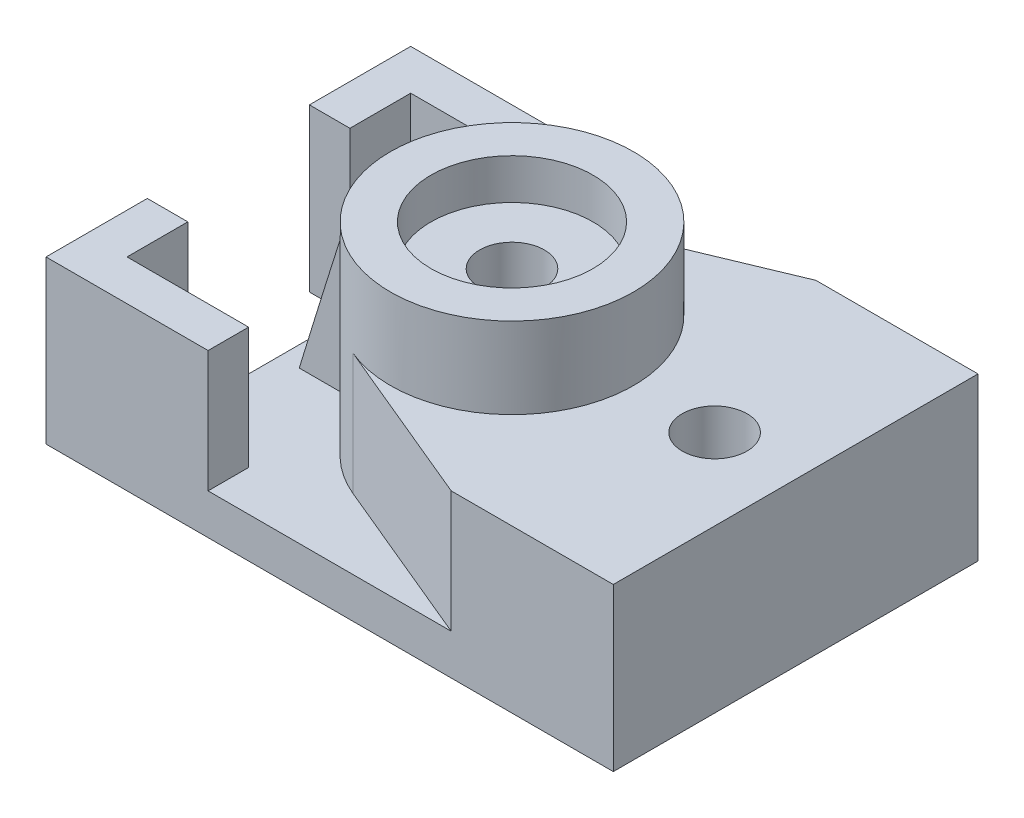
ISO-10303-21;
HEADER;
FILE_DESCRIPTION(('STEP AP214'),'2;1');
FILE_NAME('part.step','',(''),(''),'','','');
FILE_SCHEMA(('AUTOMOTIVE_DESIGN { 1 0 10303 214 1 1 1 1 }'));
ENDSEC;
DATA;
#1=APPLICATION_CONTEXT('core data for automotive mechanical design processes');
#2=APPLICATION_PROTOCOL_DEFINITION('international standard','automotive_design',2000,#1);
#3=PRODUCT_CONTEXT('',#1,'mechanical');
#4=PRODUCT('Part','Part','',(#3));
#5=PRODUCT_RELATED_PRODUCT_CATEGORY('part','',(#4));
#6=PRODUCT_DEFINITION_FORMATION('','',#4);
#7=PRODUCT_DEFINITION_CONTEXT('part definition',#1,'design');
#8=PRODUCT_DEFINITION('design','',#6,#7);
#9=PRODUCT_DEFINITION_SHAPE('','',#8);
#10=(LENGTH_UNIT() NAMED_UNIT(*) SI_UNIT(.MILLI.,.METRE.));
#11=(NAMED_UNIT(*) PLANE_ANGLE_UNIT() SI_UNIT($,.RADIAN.));
#12=(NAMED_UNIT(*) SI_UNIT($,.STERADIAN.) SOLID_ANGLE_UNIT());
#13=UNCERTAINTY_MEASURE_WITH_UNIT(LENGTH_MEASURE(1.E-05),#10,'distance_accuracy_value','');
#14=(GEOMETRIC_REPRESENTATION_CONTEXT(3) GLOBAL_UNCERTAINTY_ASSIGNED_CONTEXT((#13)) GLOBAL_UNIT_ASSIGNED_CONTEXT((#10,
#11,#12)) REPRESENTATION_CONTEXT('',''));
#15=CARTESIAN_POINT('',(0.,0.,0.));
#16=DIRECTION('',(0.,0.,1.));
#17=DIRECTION('',(1.,0.,0.));
#18=AXIS2_PLACEMENT_3D('',#15,#16,#17);
#19=CARTESIAN_POINT('',(-70.,40.,45.));
#20=DIRECTION('',(1.,0.,0.));
#21=DIRECTION('',(0.,0.,-1.));
#22=AXIS2_PLACEMENT_3D('',#19,#20,#21);
#23=PLANE('',#22);
#24=DIRECTION('',(0.,0.,1.));
#25=VECTOR('',#24,1.);
#26=CARTESIAN_POINT('',(-70.,0.,45.));
#27=LINE('',#26,#25);
#28=CARTESIAN_POINT('',(-70.,0.,-45.));
#29=VERTEX_POINT('',#28);
#30=CARTESIAN_POINT('',(-70.,0.,-20.));
#31=VERTEX_POINT('',#30);
#32=EDGE_CURVE('E422',#29,#31,#27,.T.);
#33=ORIENTED_EDGE('',*,*,#32,.T.);
#34=DIRECTION('',(0.,1.,0.));
#35=VECTOR('',#34,1.);
#36=CARTESIAN_POINT('',(-70.,10.,-20.));
#37=LINE('',#36,#35);
#38=CARTESIAN_POINT('',(-70.,40.,-20.));
#39=VERTEX_POINT('',#38);
#40=EDGE_CURVE('E365',#31,#39,#37,.T.);
#41=ORIENTED_EDGE('',*,*,#40,.T.);
#42=DIRECTION('',(0.,0.,1.));
#43=VECTOR('',#42,1.);
#44=CARTESIAN_POINT('',(-70.,40.,45.));
#45=LINE('',#44,#43);
#46=CARTESIAN_POINT('',(-70.,40.,-45.));
#47=VERTEX_POINT('',#46);
#48=EDGE_CURVE('E409',#47,#39,#45,.T.);
#49=ORIENTED_EDGE('',*,*,#48,.F.);
#50=DIRECTION('',(0.,-1.,0.));
#51=VECTOR('',#50,1.);
#52=CARTESIAN_POINT('',(-70.,40.,-45.));
#53=LINE('',#52,#51);
#54=EDGE_CURVE('E431',#47,#29,#53,.T.);
#55=ORIENTED_EDGE('',*,*,#54,.T.);
#56=EDGE_LOOP('',(#33,#41,#49,#55));
#57=FACE_BOUND('',#56,.T.);
#58=ADVANCED_FACE('F55',(#57),#23,.F.);
#59=CARTESIAN_POINT('',(0.,40.,0.));
#60=DIRECTION('',(0.,-1.,0.));
#61=DIRECTION('',(0.,0.,-1.));
#62=AXIS2_PLACEMENT_3D('',#59,#60,#61);
#63=PLANE('',#62);
#64=ORIENTED_EDGE('',*,*,#48,.T.);
#65=DIRECTION('',(-1.,0.,0.));
#66=VECTOR('',#65,1.);
#67=CARTESIAN_POINT('',(-70.,40.,-20.));
#68=LINE('',#67,#66);
#69=CARTESIAN_POINT('',(-60.,40.,-20.));
#70=VERTEX_POINT('',#69);
#71=EDGE_CURVE('E313',#70,#39,#68,.T.);
#72=ORIENTED_EDGE('',*,*,#71,.F.);
#73=DIRECTION('',(0.,0.,1.));
#74=VECTOR('',#73,1.);
#75=CARTESIAN_POINT('',(-60.,40.,-20.));
#76=LINE('',#75,#74);
#77=CARTESIAN_POINT('',(-60.,40.,-35.));
#78=VERTEX_POINT('',#77);
#79=EDGE_CURVE('E356',#78,#70,#76,.T.);
#80=ORIENTED_EDGE('',*,*,#79,.F.);
#81=DIRECTION('',(-1.,0.,0.));
#82=VECTOR('',#81,1.);
#83=CARTESIAN_POINT('',(-60.,40.,-35.));
#84=LINE('',#83,#82);
#85=CARTESIAN_POINT('',(-30.,40.,-35.));
#86=VERTEX_POINT('',#85);
#87=EDGE_CURVE('E351',#86,#78,#84,.T.);
#88=ORIENTED_EDGE('',*,*,#87,.F.);
#89=DIRECTION('',(0.,0.,1.));
#90=VECTOR('',#89,1.);
#91=CARTESIAN_POINT('',(-30.,40.,-35.));
#92=LINE('',#91,#90);
#93=CARTESIAN_POINT('',(-30.,40.,-45.));
#94=VERTEX_POINT('',#93);
#95=EDGE_CURVE('E355',#94,#86,#92,.T.);
#96=ORIENTED_EDGE('',*,*,#95,.F.);
#97=DIRECTION('',(-1.,0.,0.));
#98=VECTOR('',#97,1.);
#99=CARTESIAN_POINT('',(-70.,40.,-45.));
#100=LINE('',#99,#98);
#101=EDGE_CURVE('E405',#94,#47,#100,.T.);
#102=ORIENTED_EDGE('',*,*,#101,.T.);
#103=EDGE_LOOP('',(#64,#72,#80,#88,#96,#102));
#104=FACE_BOUND('',#103,.T.);
#105=ADVANCED_FACE('F453',(#104),#63,.F.);
#106=CARTESIAN_POINT('',(50.,40.,0.));
#107=DIRECTION('',(0.,1.,0.));
#108=DIRECTION('',(0.,0.,1.));
#109=AXIS2_PLACEMENT_3D('',#106,#107,#108);
#110=CIRCLE('',#109,8.);
#111=CARTESIAN_POINT('',(50.,40.,8.));
#112=VERTEX_POINT('',#111);
#113=EDGE_CURVE('E285',#112,#112,#110,.T.);
#114=ORIENTED_EDGE('',*,*,#113,.F.);
#115=EDGE_LOOP('',(#114));
#116=FACE_BOUND('',#115,.T.);
#117=CARTESIAN_POINT('',(70.,40.,-45.));
#118=VERTEX_POINT('',#117);
#119=CARTESIAN_POINT('',(30.,40.,-45.));
#120=VERTEX_POINT('',#119);
#121=EDGE_CURVE('E404',#118,#120,#100,.T.);
#122=ORIENTED_EDGE('',*,*,#121,.T.);
#123=DIRECTION('',(0.923076923076923,0.,-0.384615384615384));
#124=VECTOR('',#123,1.);
#125=CARTESIAN_POINT('',(-11.5384615384615,40.,-27.6923076923077));
#126=LINE('',#125,#124);
#127=CARTESIAN_POINT('',(-11.5384615384615,40.,-27.6923076923077));
#128=VERTEX_POINT('',#127);
#129=EDGE_CURVE('E348',#128,#120,#126,.T.);
#130=ORIENTED_EDGE('',*,*,#129,.F.);
#131=CARTESIAN_POINT('',(0.,40.,0.));
#132=DIRECTION('',(0.,-1.,0.));
#133=DIRECTION('',(0.,0.,-1.));
#134=AXIS2_PLACEMENT_3D('',#131,#132,#133);
#135=CIRCLE('',#134,30.);
#136=CARTESIAN_POINT('',(-11.5384615384615,40.,27.6923076923077));
#137=VERTEX_POINT('',#136);
#138=EDGE_CURVE('E393',#137,#128,#135,.F.);
#139=ORIENTED_EDGE('',*,*,#138,.F.);
#140=DIRECTION('',(-0.923076923076923,0.,-0.384615384615384));
#141=VECTOR('',#140,1.);
#142=CARTESIAN_POINT('',(-11.5384615384615,40.,27.6923076923077));
#143=LINE('',#142,#141);
#144=CARTESIAN_POINT('',(30.,40.,45.));
#145=VERTEX_POINT('',#144);
#146=EDGE_CURVE('E349',#145,#137,#143,.T.);
#147=ORIENTED_EDGE('',*,*,#146,.F.);
#148=DIRECTION('',(1.,0.,0.));
#149=VECTOR('',#148,1.);
#150=CARTESIAN_POINT('',(-70.,40.,45.));
#151=LINE('',#150,#149);
#152=CARTESIAN_POINT('',(70.,40.,45.));
#153=VERTEX_POINT('',#152);
#154=EDGE_CURVE('E412',#145,#153,#151,.T.);
#155=ORIENTED_EDGE('',*,*,#154,.T.);
#156=DIRECTION('',(0.,0.,-1.));
#157=VECTOR('',#156,1.);
#158=CARTESIAN_POINT('',(70.,40.,45.));
#159=LINE('',#158,#157);
#160=EDGE_CURVE('E399',#153,#118,#159,.T.);
#161=ORIENTED_EDGE('',*,*,#160,.T.);
#162=EDGE_LOOP('',(#122,#130,#139,#147,#155,#161));
#163=FACE_BOUND('',#162,.T.);
#164=ADVANCED_FACE('F467',(#116,#163),#63,.F.);
#165=CARTESIAN_POINT('',(70.,40.,45.));
#166=DIRECTION('',(-1.,0.,0.));
#167=DIRECTION('',(0.,0.,1.));
#168=AXIS2_PLACEMENT_3D('',#165,#166,#167);
#169=PLANE('',#168);
#170=DIRECTION('',(0.,0.,-1.));
#171=VECTOR('',#170,1.);
#172=CARTESIAN_POINT('',(70.,0.,45.));
#173=LINE('',#172,#171);
#174=CARTESIAN_POINT('',(70.,0.,45.));
#175=VERTEX_POINT('',#174);
#176=CARTESIAN_POINT('',(70.,0.,-45.));
#177=VERTEX_POINT('',#176);
#178=EDGE_CURVE('E417',#175,#177,#173,.T.);
#179=ORIENTED_EDGE('',*,*,#178,.T.);
#180=DIRECTION('',(0.,-1.,0.));
#181=VECTOR('',#180,1.);
#182=CARTESIAN_POINT('',(70.,40.,-45.));
#183=LINE('',#182,#181);
#184=EDGE_CURVE('E398',#118,#177,#183,.T.);
#185=ORIENTED_EDGE('',*,*,#184,.F.);
#186=ORIENTED_EDGE('',*,*,#160,.F.);
#187=DIRECTION('',(0.,-1.,0.));
#188=VECTOR('',#187,1.);
#189=CARTESIAN_POINT('',(70.,40.,45.));
#190=LINE('',#189,#188);
#191=EDGE_CURVE('E413',#153,#175,#190,.T.);
#192=ORIENTED_EDGE('',*,*,#191,.T.);
#193=EDGE_LOOP('',(#179,#185,#186,#192));
#194=FACE_BOUND('',#193,.T.);
#195=ADVANCED_FACE('F53',(#194),#169,.F.);
#196=CARTESIAN_POINT('',(-70.,40.,-45.));
#197=DIRECTION('',(0.,0.,1.));
#198=DIRECTION('',(1.,0.,0.));
#199=AXIS2_PLACEMENT_3D('',#196,#197,#198);
#200=PLANE('',#199);
#201=ORIENTED_EDGE('',*,*,#101,.F.);
#202=DIRECTION('',(0.,1.,0.));
#203=VECTOR('',#202,1.);
#204=CARTESIAN_POINT('',(-30.,10.,-45.));
#205=LINE('',#204,#203);
#206=CARTESIAN_POINT('',(-30.,10.,-45.));
#207=VERTEX_POINT('',#206);
#208=EDGE_CURVE('E375',#207,#94,#205,.T.);
#209=ORIENTED_EDGE('',*,*,#208,.F.);
#210=DIRECTION('',(-1.,0.,0.));
#211=VECTOR('',#210,1.);
#212=CARTESIAN_POINT('',(-30.,10.,-45.));
#213=LINE('',#212,#211);
#214=CARTESIAN_POINT('',(30.,10.,-45.));
#215=VERTEX_POINT('',#214);
#216=EDGE_CURVE('E323',#215,#207,#213,.T.);
#217=ORIENTED_EDGE('',*,*,#216,.F.);
#218=DIRECTION('',(0.,1.,0.));
#219=VECTOR('',#218,1.);
#220=CARTESIAN_POINT('',(30.,10.,-45.));
#221=LINE('',#220,#219);
#222=EDGE_CURVE('E372',#215,#120,#221,.T.);
#223=ORIENTED_EDGE('',*,*,#222,.T.);
#224=ORIENTED_EDGE('',*,*,#121,.F.);
#225=ORIENTED_EDGE('',*,*,#184,.T.);
#226=DIRECTION('',(-1.,0.,0.));
#227=VECTOR('',#226,1.);
#228=CARTESIAN_POINT('',(-70.,0.,-45.));
#229=LINE('',#228,#227);
#230=EDGE_CURVE('E419',#177,#29,#229,.T.);
#231=ORIENTED_EDGE('',*,*,#230,.T.);
#232=ORIENTED_EDGE('',*,*,#54,.F.);
#233=EDGE_LOOP('',(#201,#209,#217,#223,#224,#225,#231,#232));
#234=FACE_BOUND('',#233,.T.);
#235=ADVANCED_FACE('F440',(#234),#200,.F.);
#236=DIRECTION('',(0.,1.,0.));
#237=VECTOR('',#236,1.);
#238=CARTESIAN_POINT('',(-70.,10.,20.));
#239=LINE('',#238,#237);
#240=CARTESIAN_POINT('',(-70.,0.,20.));
#241=VERTEX_POINT('',#240);
#242=CARTESIAN_POINT('',(-70.,40.,20.));
#243=VERTEX_POINT('',#242);
#244=EDGE_CURVE('E340',#241,#243,#239,.T.);
#245=ORIENTED_EDGE('',*,*,#244,.F.);
#246=CARTESIAN_POINT('',(-70.,0.,45.));
#247=VERTEX_POINT('',#246);
#248=EDGE_CURVE('E423',#241,#247,#27,.T.);
#249=ORIENTED_EDGE('',*,*,#248,.T.);
#250=DIRECTION('',(0.,-1.,0.));
#251=VECTOR('',#250,1.);
#252=CARTESIAN_POINT('',(-70.,40.,45.));
#253=LINE('',#252,#251);
#254=CARTESIAN_POINT('',(-70.,40.,45.));
#255=VERTEX_POINT('',#254);
#256=EDGE_CURVE('E426',#255,#247,#253,.T.);
#257=ORIENTED_EDGE('',*,*,#256,.F.);
#258=EDGE_CURVE('E410',#243,#255,#45,.T.);
#259=ORIENTED_EDGE('',*,*,#258,.F.);
#260=EDGE_LOOP('',(#245,#249,#257,#259));
#261=FACE_BOUND('',#260,.T.);
#262=ADVANCED_FACE('F480',(#261),#23,.F.);
#263=CARTESIAN_POINT('',(-70.,40.,45.));
#264=DIRECTION('',(0.,0.,-1.));
#265=DIRECTION('',(-1.,0.,0.));
#266=AXIS2_PLACEMENT_3D('',#263,#264,#265);
#267=PLANE('',#266);
#268=ORIENTED_EDGE('',*,*,#154,.F.);
#269=DIRECTION('',(0.,1.,0.));
#270=VECTOR('',#269,1.);
#271=CARTESIAN_POINT('',(30.,10.,45.));
#272=LINE('',#271,#270);
#273=CARTESIAN_POINT('',(30.,10.,45.));
#274=VERTEX_POINT('',#273);
#275=EDGE_CURVE('E382',#274,#145,#272,.T.);
#276=ORIENTED_EDGE('',*,*,#275,.F.);
#277=DIRECTION('',(1.,0.,0.));
#278=VECTOR('',#277,1.);
#279=CARTESIAN_POINT('',(-30.,10.,45.));
#280=LINE('',#279,#278);
#281=CARTESIAN_POINT('',(-30.,10.,45.));
#282=VERTEX_POINT('',#281);
#283=EDGE_CURVE('E318',#282,#274,#280,.T.);
#284=ORIENTED_EDGE('',*,*,#283,.F.);
#285=DIRECTION('',(0.,1.,0.));
#286=VECTOR('',#285,1.);
#287=CARTESIAN_POINT('',(-30.,10.,45.));
#288=LINE('',#287,#286);
#289=CARTESIAN_POINT('',(-30.,40.,45.));
#290=VERTEX_POINT('',#289);
#291=EDGE_CURVE('E384',#282,#290,#288,.T.);
#292=ORIENTED_EDGE('',*,*,#291,.T.);
#293=EDGE_CURVE('E415',#255,#290,#151,.T.);
#294=ORIENTED_EDGE('',*,*,#293,.F.);
#295=ORIENTED_EDGE('',*,*,#256,.T.);
#296=DIRECTION('',(1.,0.,0.));
#297=VECTOR('',#296,1.);
#298=CARTESIAN_POINT('',(-70.,0.,45.));
#299=LINE('',#298,#297);
#300=EDGE_CURVE('E401',#247,#175,#299,.T.);
#301=ORIENTED_EDGE('',*,*,#300,.T.);
#302=ORIENTED_EDGE('',*,*,#191,.F.);
#303=EDGE_LOOP('',(#268,#276,#284,#292,#294,#295,#301,#302));
#304=FACE_BOUND('',#303,.T.);
#305=ADVANCED_FACE('F475',(#304),#267,.F.);
#306=ORIENTED_EDGE('',*,*,#293,.T.);
#307=DIRECTION('',(0.,0.,1.));
#308=VECTOR('',#307,1.);
#309=CARTESIAN_POINT('',(-30.,40.,35.));
#310=LINE('',#309,#308);
#311=CARTESIAN_POINT('',(-30.,40.,35.));
#312=VERTEX_POINT('',#311);
#313=EDGE_CURVE('E347',#312,#290,#310,.T.);
#314=ORIENTED_EDGE('',*,*,#313,.F.);
#315=DIRECTION('',(1.,0.,0.));
#316=VECTOR('',#315,1.);
#317=CARTESIAN_POINT('',(-60.,40.,35.));
#318=LINE('',#317,#316);
#319=CARTESIAN_POINT('',(-60.,40.,35.));
#320=VERTEX_POINT('',#319);
#321=EDGE_CURVE('E344',#320,#312,#318,.T.);
#322=ORIENTED_EDGE('',*,*,#321,.F.);
#323=DIRECTION('',(0.,0.,1.));
#324=VECTOR('',#323,1.);
#325=CARTESIAN_POINT('',(-60.,40.,20.));
#326=LINE('',#325,#324);
#327=CARTESIAN_POINT('',(-60.,40.,20.));
#328=VERTEX_POINT('',#327);
#329=EDGE_CURVE('E338',#328,#320,#326,.T.);
#330=ORIENTED_EDGE('',*,*,#329,.F.);
#331=DIRECTION('',(1.,0.,0.));
#332=VECTOR('',#331,1.);
#333=CARTESIAN_POINT('',(-70.,40.,20.));
#334=LINE('',#333,#332);
#335=EDGE_CURVE('E307',#243,#328,#334,.T.);
#336=ORIENTED_EDGE('',*,*,#335,.F.);
#337=ORIENTED_EDGE('',*,*,#258,.T.);
#338=EDGE_LOOP('',(#306,#314,#322,#330,#336,#337));
#339=FACE_BOUND('',#338,.T.);
#340=ADVANCED_FACE('F513',(#339),#63,.F.);
#341=CARTESIAN_POINT('',(0.,0.,0.));
#342=DIRECTION('',(0.,-1.,0.));
#343=DIRECTION('',(0.,0.,-1.));
#344=AXIS2_PLACEMENT_3D('',#341,#342,#343);
#345=PLANE('',#344);
#346=DIRECTION('',(-1.,0.,0.));
#347=VECTOR('',#346,1.);
#348=CARTESIAN_POINT('',(-70.,0.,-20.));
#349=LINE('',#348,#347);
#350=CARTESIAN_POINT('',(-50.,0.,-20.));
#351=VERTEX_POINT('',#350);
#352=EDGE_CURVE('E295',#351,#31,#349,.T.);
#353=ORIENTED_EDGE('',*,*,#352,.T.);
#354=ORIENTED_EDGE('',*,*,#32,.F.);
#355=ORIENTED_EDGE('',*,*,#230,.F.);
#356=ORIENTED_EDGE('',*,*,#178,.F.);
#357=ORIENTED_EDGE('',*,*,#300,.F.);
#358=ORIENTED_EDGE('',*,*,#248,.F.);
#359=DIRECTION('',(1.,0.,0.));
#360=VECTOR('',#359,1.);
#361=CARTESIAN_POINT('',(-70.,0.,20.));
#362=LINE('',#361,#360);
#363=CARTESIAN_POINT('',(-50.,0.,20.));
#364=VERTEX_POINT('',#363);
#365=EDGE_CURVE('E288',#241,#364,#362,.T.);
#366=ORIENTED_EDGE('',*,*,#365,.T.);
#367=DIRECTION('',(0.,0.,-1.));
#368=VECTOR('',#367,1.);
#369=CARTESIAN_POINT('',(-50.,0.,-20.));
#370=LINE('',#369,#368);
#371=EDGE_CURVE('E293',#364,#351,#370,.T.);
#372=ORIENTED_EDGE('',*,*,#371,.T.);
#373=EDGE_LOOP('',(#353,#354,#355,#356,#357,#358,#366,#372));
#374=FACE_BOUND('',#373,.T.);
#375=CARTESIAN_POINT('',(50.,0.,0.));
#376=DIRECTION('',(0.,-1.,0.));
#377=DIRECTION('',(0.,0.,-1.));
#378=AXIS2_PLACEMENT_3D('',#375,#376,#377);
#379=CIRCLE('',#378,8.);
#380=CARTESIAN_POINT('',(50.,0.,-8.));
#381=VERTEX_POINT('',#380);
#382=EDGE_CURVE('E287',#381,#381,#379,.F.);
#383=ORIENTED_EDGE('',*,*,#382,.T.);
#384=EDGE_LOOP('',(#383));
#385=FACE_BOUND('',#384,.T.);
#386=CARTESIAN_POINT('',(0.,0.,0.));
#387=DIRECTION('',(0.,-1.,0.));
#388=DIRECTION('',(0.,0.,-1.));
#389=AXIS2_PLACEMENT_3D('',#386,#387,#388);
#390=CIRCLE('',#389,8.);
#391=CARTESIAN_POINT('',(0.,0.,-8.));
#392=VERTEX_POINT('',#391);
#393=EDGE_CURVE('E283',#392,#392,#390,.F.);
#394=ORIENTED_EDGE('',*,*,#393,.T.);
#395=EDGE_LOOP('',(#394));
#396=FACE_BOUND('',#395,.T.);
#397=ADVANCED_FACE('F444',(#374,#385,#396),#345,.T.);
#398=CARTESIAN_POINT('',(0.,60.,0.));
#399=DIRECTION('',(0.,-1.,0.));
#400=DIRECTION('',(0.,0.,-1.));
#401=AXIS2_PLACEMENT_3D('',#398,#399,#400);
#402=CYLINDRICAL_SURFACE('',#401,30.);
#403=CARTESIAN_POINT('',(0.,60.,0.));
#404=DIRECTION('',(0.,1.,0.));
#405=DIRECTION('',(0.,0.,1.));
#406=AXIS2_PLACEMENT_3D('',#403,#404,#405);
#407=CIRCLE('',#406,30.);
#408=CARTESIAN_POINT('',(-29.0473750965556,60.,7.5));
#409=VERTEX_POINT('',#408);
#410=CARTESIAN_POINT('',(-29.0473750965556,60.,-7.5));
#411=VERTEX_POINT('',#410);
#412=EDGE_CURVE('E220',#409,#411,#407,.T.);
#413=ORIENTED_EDGE('',*,*,#412,.F.);
#414=DIRECTION('',(0.,1.,0.));
#415=VECTOR('',#414,1.);
#416=CARTESIAN_POINT('',(-29.0473750965556,-11.8971742768329,7.5));
#417=LINE('',#416,#415);
#418=CARTESIAN_POINT('',(-29.0473750965556,10.,7.5));
#419=VERTEX_POINT('',#418);
#420=EDGE_CURVE('E209',#419,#409,#417,.T.);
#421=ORIENTED_EDGE('',*,*,#420,.F.);
#422=CARTESIAN_POINT('',(0.,10.,0.));
#423=DIRECTION('',(0.,-1.,0.));
#424=DIRECTION('',(0.,0.,1.));
#425=AXIS2_PLACEMENT_3D('',#422,#423,#424);
#426=CIRCLE('',#425,30.);
#427=CARTESIAN_POINT('',(-11.5384615384615,10.,27.6923076923077));
#428=VERTEX_POINT('',#427);
#429=EDGE_CURVE('E214',#428,#419,#426,.T.);
#430=ORIENTED_EDGE('',*,*,#429,.F.);
#431=DIRECTION('',(0.,1.,0.));
#432=VECTOR('',#431,1.);
#433=CARTESIAN_POINT('',(-11.5384615384615,10.,27.6923076923077));
#434=LINE('',#433,#432);
#435=EDGE_CURVE('E378',#428,#137,#434,.T.);
#436=ORIENTED_EDGE('',*,*,#435,.T.);
#437=ORIENTED_EDGE('',*,*,#138,.T.);
#438=DIRECTION('',(0.,1.,0.));
#439=VECTOR('',#438,1.);
#440=CARTESIAN_POINT('',(-11.5384615384615,10.,-27.6923076923077));
#441=LINE('',#440,#439);
#442=CARTESIAN_POINT('',(-11.5384615384615,10.,-27.6923076923077));
#443=VERTEX_POINT('',#442);
#444=EDGE_CURVE('E380',#443,#128,#441,.T.);
#445=ORIENTED_EDGE('',*,*,#444,.F.);
#446=CARTESIAN_POINT('',(-29.0473750965556,10.,-7.5));
#447=VERTEX_POINT('',#446);
#448=EDGE_CURVE('E230',#447,#443,#426,.T.);
#449=ORIENTED_EDGE('',*,*,#448,.F.);
#450=DIRECTION('',(0.,1.,0.));
#451=VECTOR('',#450,1.);
#452=CARTESIAN_POINT('',(-29.0473750965556,-11.8971742768329,-7.5));
#453=LINE('',#452,#451);
#454=EDGE_CURVE('E218',#447,#411,#453,.T.);
#455=ORIENTED_EDGE('',*,*,#454,.T.);
#456=EDGE_LOOP('',(#413,#421,#430,#436,#437,#445,#449,#455));
#457=FACE_BOUND('',#456,.T.);
#458=ADVANCED_FACE('F212',(#457),#402,.T.);
#459=CARTESIAN_POINT('',(0.,60.,0.));
#460=DIRECTION('',(0.,-1.,0.));
#461=DIRECTION('',(0.,0.,-1.));
#462=AXIS2_PLACEMENT_3D('',#459,#460,#461);
#463=CYLINDRICAL_SURFACE('',#462,20.);
#464=CARTESIAN_POINT('',(0.,50.,0.));
#465=DIRECTION('',(0.,1.,0.));
#466=DIRECTION('',(0.,0.,1.));
#467=AXIS2_PLACEMENT_3D('',#464,#465,#466);
#468=CIRCLE('',#467,20.);
#469=CARTESIAN_POINT('',(0.,50.,20.));
#470=VERTEX_POINT('',#469);
#471=EDGE_CURVE('E12',#470,#470,#468,.T.);
#472=ORIENTED_EDGE('',*,*,#471,.F.);
#473=EDGE_LOOP('',(#472));
#474=FACE_BOUND('',#473,.T.);
#475=CARTESIAN_POINT('',(0.,60.,0.));
#476=DIRECTION('',(0.,1.,0.));
#477=DIRECTION('',(0.,0.,1.));
#478=AXIS2_PLACEMENT_3D('',#475,#476,#477);
#479=CIRCLE('',#478,20.);
#480=CARTESIAN_POINT('',(0.,60.,20.));
#481=VERTEX_POINT('',#480);
#482=EDGE_CURVE('E362',#481,#481,#479,.T.);
#483=ORIENTED_EDGE('',*,*,#482,.T.);
#484=EDGE_LOOP('',(#483));
#485=FACE_BOUND('',#484,.T.);
#486=ADVANCED_FACE('F567',(#474,#485),#463,.F.);
#487=CARTESIAN_POINT('',(0.,60.,0.));
#488=DIRECTION('',(0.,1.,0.));
#489=DIRECTION('',(0.,0.,1.));
#490=AXIS2_PLACEMENT_3D('',#487,#488,#489);
#491=PLANE('',#490);
#492=CARTESIAN_POINT('',(0.,60.,0.));
#493=DIRECTION('',(0.,-1.,0.));
#494=DIRECTION('',(0.,0.,1.));
#495=AXIS2_PLACEMENT_3D('',#492,#493,#494);
#496=CIRCLE('',#495,30.);
#497=EDGE_CURVE('E66',#409,#411,#496,.T.);
#498=ORIENTED_EDGE('',*,*,#497,.F.);
#499=ORIENTED_EDGE('',*,*,#412,.T.);
#500=EDGE_LOOP('',(#498,#499));
#501=FACE_BOUND('',#500,.T.);
#502=ORIENTED_EDGE('',*,*,#482,.F.);
#503=EDGE_LOOP('',(#502));
#504=FACE_BOUND('',#503,.T.);
#505=ADVANCED_FACE('F575',(#501,#504),#491,.T.);
#506=CARTESIAN_POINT('',(-70.,10.,-20.));
#507=DIRECTION('',(0.,0.,-1.));
#508=DIRECTION('',(-1.,0.,0.));
#509=AXIS2_PLACEMENT_3D('',#506,#507,#508);
#510=PLANE('',#509);
#511=ORIENTED_EDGE('',*,*,#71,.T.);
#512=ORIENTED_EDGE('',*,*,#40,.F.);
#513=ORIENTED_EDGE('',*,*,#352,.F.);
#514=DIRECTION('',(0.,1.,0.));
#515=VECTOR('',#514,1.);
#516=CARTESIAN_POINT('',(-50.,-0.001000000000001,-20.));
#517=LINE('',#516,#515);
#518=CARTESIAN_POINT('',(-50.,10.,-20.));
#519=VERTEX_POINT('',#518);
#520=EDGE_CURVE('E296',#351,#519,#517,.T.);
#521=ORIENTED_EDGE('',*,*,#520,.T.);
#522=DIRECTION('',(-1.,0.,0.));
#523=VECTOR('',#522,1.);
#524=CARTESIAN_POINT('',(0.,10.,-20.));
#525=LINE('',#524,#523);
#526=CARTESIAN_POINT('',(-60.,10.,-20.));
#527=VERTEX_POINT('',#526);
#528=EDGE_CURVE('E239',#519,#527,#525,.T.);
#529=ORIENTED_EDGE('',*,*,#528,.T.);
#530=DIRECTION('',(0.,1.,0.));
#531=VECTOR('',#530,1.);
#532=CARTESIAN_POINT('',(-60.,10.,-20.));
#533=LINE('',#532,#531);
#534=EDGE_CURVE('E366',#527,#70,#533,.T.);
#535=ORIENTED_EDGE('',*,*,#534,.T.);
#536=EDGE_LOOP('',(#511,#512,#513,#521,#529,#535));
#537=FACE_BOUND('',#536,.T.);
#538=ADVANCED_FACE('F489',(#537),#510,.F.);
#539=CARTESIAN_POINT('',(-60.,10.,-20.));
#540=DIRECTION('',(-1.,0.,0.));
#541=DIRECTION('',(0.,0.,1.));
#542=AXIS2_PLACEMENT_3D('',#539,#540,#541);
#543=PLANE('',#542);
#544=ORIENTED_EDGE('',*,*,#79,.T.);
#545=ORIENTED_EDGE('',*,*,#534,.F.);
#546=DIRECTION('',(0.,0.,1.));
#547=VECTOR('',#546,1.);
#548=CARTESIAN_POINT('',(-60.,10.,-20.));
#549=LINE('',#548,#547);
#550=CARTESIAN_POINT('',(-60.,10.,-35.));
#551=VERTEX_POINT('',#550);
#552=EDGE_CURVE('E334',#551,#527,#549,.T.);
#553=ORIENTED_EDGE('',*,*,#552,.F.);
#554=DIRECTION('',(0.,1.,0.));
#555=VECTOR('',#554,1.);
#556=CARTESIAN_POINT('',(-60.,10.,-35.));
#557=LINE('',#556,#555);
#558=EDGE_CURVE('E368',#551,#78,#557,.T.);
#559=ORIENTED_EDGE('',*,*,#558,.T.);
#560=EDGE_LOOP('',(#544,#545,#553,#559));
#561=FACE_BOUND('',#560,.T.);
#562=ADVANCED_FACE('F494',(#561),#543,.F.);
#563=CARTESIAN_POINT('',(-60.,10.,-35.));
#564=DIRECTION('',(0.,0.,-1.));
#565=DIRECTION('',(-1.,0.,0.));
#566=AXIS2_PLACEMENT_3D('',#563,#564,#565);
#567=PLANE('',#566);
#568=ORIENTED_EDGE('',*,*,#87,.T.);
#569=ORIENTED_EDGE('',*,*,#558,.F.);
#570=DIRECTION('',(-1.,0.,0.));
#571=VECTOR('',#570,1.);
#572=CARTESIAN_POINT('',(-60.,10.,-35.));
#573=LINE('',#572,#571);
#574=CARTESIAN_POINT('',(-30.,10.,-35.));
#575=VERTEX_POINT('',#574);
#576=EDGE_CURVE('E332',#575,#551,#573,.T.);
#577=ORIENTED_EDGE('',*,*,#576,.F.);
#578=DIRECTION('',(0.,1.,0.));
#579=VECTOR('',#578,1.);
#580=CARTESIAN_POINT('',(-30.,10.,-35.));
#581=LINE('',#580,#579);
#582=EDGE_CURVE('E369',#575,#86,#581,.T.);
#583=ORIENTED_EDGE('',*,*,#582,.T.);
#584=EDGE_LOOP('',(#568,#569,#577,#583));
#585=FACE_BOUND('',#584,.T.);
#586=ADVANCED_FACE('F496',(#585),#567,.F.);
#587=CARTESIAN_POINT('',(-30.,10.,-35.));
#588=DIRECTION('',(-1.,0.,0.));
#589=DIRECTION('',(0.,0.,1.));
#590=AXIS2_PLACEMENT_3D('',#587,#588,#589);
#591=PLANE('',#590);
#592=ORIENTED_EDGE('',*,*,#95,.T.);
#593=ORIENTED_EDGE('',*,*,#582,.F.);
#594=DIRECTION('',(0.,0.,1.));
#595=VECTOR('',#594,1.);
#596=CARTESIAN_POINT('',(-30.,10.,-35.));
#597=LINE('',#596,#595);
#598=EDGE_CURVE('E329',#207,#575,#597,.T.);
#599=ORIENTED_EDGE('',*,*,#598,.F.);
#600=ORIENTED_EDGE('',*,*,#208,.T.);
#601=EDGE_LOOP('',(#592,#593,#599,#600));
#602=FACE_BOUND('',#601,.T.);
#603=ADVANCED_FACE('F458',(#602),#591,.F.);
#604=CARTESIAN_POINT('',(-11.5384615384615,10.,-27.6923076923077));
#605=DIRECTION('',(0.384615384615384,0.,0.923076923076923));
#606=DIRECTION('',(0.923076923076923,0.,-0.384615384615384));
#607=AXIS2_PLACEMENT_3D('',#604,#605,#606);
#608=PLANE('',#607);
#609=ORIENTED_EDGE('',*,*,#129,.T.);
#610=ORIENTED_EDGE('',*,*,#222,.F.);
#611=DIRECTION('',(0.923076923076923,0.,-0.384615384615384));
#612=VECTOR('',#611,1.);
#613=CARTESIAN_POINT('',(-11.5384615384615,10.,-27.6923076923077));
#614=LINE('',#613,#612);
#615=EDGE_CURVE('E226',#443,#215,#614,.T.);
#616=ORIENTED_EDGE('',*,*,#615,.F.);
#617=ORIENTED_EDGE('',*,*,#444,.T.);
#618=EDGE_LOOP('',(#609,#610,#616,#617));
#619=FACE_BOUND('',#618,.T.);
#620=ADVANCED_FACE('F503',(#619),#608,.F.);
#621=CARTESIAN_POINT('',(-11.5384615384615,10.,27.6923076923077));
#622=DIRECTION('',(0.384615384615384,0.,-0.923076923076923));
#623=DIRECTION('',(-0.923076923076923,0.,-0.384615384615384));
#624=AXIS2_PLACEMENT_3D('',#621,#622,#623);
#625=PLANE('',#624);
#626=ORIENTED_EDGE('',*,*,#146,.T.);
#627=ORIENTED_EDGE('',*,*,#435,.F.);
#628=DIRECTION('',(-0.923076923076923,0.,-0.384615384615384));
#629=VECTOR('',#628,1.);
#630=CARTESIAN_POINT('',(-11.5384615384615,10.,27.6923076923077));
#631=LINE('',#630,#629);
#632=EDGE_CURVE('E227',#274,#428,#631,.T.);
#633=ORIENTED_EDGE('',*,*,#632,.F.);
#634=ORIENTED_EDGE('',*,*,#275,.T.);
#635=EDGE_LOOP('',(#626,#627,#633,#634));
#636=FACE_BOUND('',#635,.T.);
#637=ADVANCED_FACE('F553',(#636),#625,.F.);
#638=CARTESIAN_POINT('',(-30.,10.,35.));
#639=DIRECTION('',(-1.,0.,0.));
#640=DIRECTION('',(0.,0.,1.));
#641=AXIS2_PLACEMENT_3D('',#638,#639,#640);
#642=PLANE('',#641);
#643=ORIENTED_EDGE('',*,*,#313,.T.);
#644=ORIENTED_EDGE('',*,*,#291,.F.);
#645=DIRECTION('',(0.,0.,1.));
#646=VECTOR('',#645,1.);
#647=CARTESIAN_POINT('',(-30.,10.,35.));
#648=LINE('',#647,#646);
#649=CARTESIAN_POINT('',(-30.,10.,35.));
#650=VERTEX_POINT('',#649);
#651=EDGE_CURVE('E320',#650,#282,#648,.T.);
#652=ORIENTED_EDGE('',*,*,#651,.F.);
#653=DIRECTION('',(0.,1.,0.));
#654=VECTOR('',#653,1.);
#655=CARTESIAN_POINT('',(-30.,10.,35.));
#656=LINE('',#655,#654);
#657=EDGE_CURVE('E387',#650,#312,#656,.T.);
#658=ORIENTED_EDGE('',*,*,#657,.T.);
#659=EDGE_LOOP('',(#643,#644,#652,#658));
#660=FACE_BOUND('',#659,.T.);
#661=ADVANCED_FACE('F549',(#660),#642,.F.);
#662=CARTESIAN_POINT('',(-60.,10.,35.));
#663=DIRECTION('',(0.,0.,1.));
#664=DIRECTION('',(1.,0.,0.));
#665=AXIS2_PLACEMENT_3D('',#662,#663,#664);
#666=PLANE('',#665);
#667=ORIENTED_EDGE('',*,*,#321,.T.);
#668=ORIENTED_EDGE('',*,*,#657,.F.);
#669=DIRECTION('',(1.,0.,0.));
#670=VECTOR('',#669,1.);
#671=CARTESIAN_POINT('',(-60.,10.,35.));
#672=LINE('',#671,#670);
#673=CARTESIAN_POINT('',(-60.,10.,35.));
#674=VERTEX_POINT('',#673);
#675=EDGE_CURVE('E312',#674,#650,#672,.T.);
#676=ORIENTED_EDGE('',*,*,#675,.F.);
#677=DIRECTION('',(0.,1.,0.));
#678=VECTOR('',#677,1.);
#679=CARTESIAN_POINT('',(-60.,10.,35.));
#680=LINE('',#679,#678);
#681=EDGE_CURVE('E389',#674,#320,#680,.T.);
#682=ORIENTED_EDGE('',*,*,#681,.T.);
#683=EDGE_LOOP('',(#667,#668,#676,#682));
#684=FACE_BOUND('',#683,.T.);
#685=ADVANCED_FACE('F550',(#684),#666,.F.);
#686=CARTESIAN_POINT('',(-60.,10.,20.));
#687=DIRECTION('',(-1.,0.,0.));
#688=DIRECTION('',(0.,0.,1.));
#689=AXIS2_PLACEMENT_3D('',#686,#687,#688);
#690=PLANE('',#689);
#691=ORIENTED_EDGE('',*,*,#329,.T.);
#692=ORIENTED_EDGE('',*,*,#681,.F.);
#693=DIRECTION('',(0.,0.,1.));
#694=VECTOR('',#693,1.);
#695=CARTESIAN_POINT('',(-60.,10.,20.));
#696=LINE('',#695,#694);
#697=CARTESIAN_POINT('',(-60.,10.,20.));
#698=VERTEX_POINT('',#697);
#699=EDGE_CURVE('E309',#698,#674,#696,.T.);
#700=ORIENTED_EDGE('',*,*,#699,.F.);
#701=DIRECTION('',(0.,1.,0.));
#702=VECTOR('',#701,1.);
#703=CARTESIAN_POINT('',(-60.,10.,20.));
#704=LINE('',#703,#702);
#705=EDGE_CURVE('E388',#698,#328,#704,.T.);
#706=ORIENTED_EDGE('',*,*,#705,.T.);
#707=EDGE_LOOP('',(#691,#692,#700,#706));
#708=FACE_BOUND('',#707,.T.);
#709=ADVANCED_FACE('F545',(#708),#690,.F.);
#710=CARTESIAN_POINT('',(-70.,10.,20.));
#711=DIRECTION('',(0.,0.,1.));
#712=DIRECTION('',(1.,0.,0.));
#713=AXIS2_PLACEMENT_3D('',#710,#711,#712);
#714=PLANE('',#713);
#715=ORIENTED_EDGE('',*,*,#335,.T.);
#716=ORIENTED_EDGE('',*,*,#705,.F.);
#717=DIRECTION('',(-1.,0.,0.));
#718=VECTOR('',#717,1.);
#719=CARTESIAN_POINT('',(-70.,10.,20.));
#720=LINE('',#719,#718);
#721=CARTESIAN_POINT('',(-50.,10.,20.));
#722=VERTEX_POINT('',#721);
#723=EDGE_CURVE('E301',#722,#698,#720,.T.);
#724=ORIENTED_EDGE('',*,*,#723,.F.);
#725=DIRECTION('',(0.,1.,0.));
#726=VECTOR('',#725,1.);
#727=CARTESIAN_POINT('',(-50.,-0.001000000000001,20.));
#728=LINE('',#727,#726);
#729=EDGE_CURVE('E300',#364,#722,#728,.T.);
#730=ORIENTED_EDGE('',*,*,#729,.F.);
#731=ORIENTED_EDGE('',*,*,#365,.F.);
#732=ORIENTED_EDGE('',*,*,#244,.T.);
#733=EDGE_LOOP('',(#715,#716,#724,#730,#731,#732));
#734=FACE_BOUND('',#733,.T.);
#735=ADVANCED_FACE('F482',(#734),#714,.F.);
#736=CARTESIAN_POINT('',(0.,10.,0.));
#737=DIRECTION('',(0.,1.,0.));
#738=DIRECTION('',(0.,0.,1.));
#739=AXIS2_PLACEMENT_3D('',#736,#737,#738);
#740=PLANE('',#739);
#741=DIRECTION('',(0.,0.,1.));
#742=VECTOR('',#741,1.);
#743=CARTESIAN_POINT('',(-50.,10.,-20.));
#744=LINE('',#743,#742);
#745=EDGE_CURVE('E234',#519,#722,#744,.T.);
#746=ORIENTED_EDGE('',*,*,#745,.T.);
#747=ORIENTED_EDGE('',*,*,#723,.T.);
#748=ORIENTED_EDGE('',*,*,#699,.T.);
#749=ORIENTED_EDGE('',*,*,#675,.T.);
#750=ORIENTED_EDGE('',*,*,#651,.T.);
#751=ORIENTED_EDGE('',*,*,#283,.T.);
#752=ORIENTED_EDGE('',*,*,#632,.T.);
#753=ORIENTED_EDGE('',*,*,#429,.T.);
#754=DIRECTION('',(-1.,0.,0.));
#755=VECTOR('',#754,1.);
#756=CARTESIAN_POINT('',(-29.0473750965556,10.,7.5));
#757=LINE('',#756,#755);
#758=CARTESIAN_POINT('',(-45.,10.,7.5));
#759=VERTEX_POINT('',#758);
#760=EDGE_CURVE('E221',#419,#759,#757,.T.);
#761=ORIENTED_EDGE('',*,*,#760,.T.);
#762=DIRECTION('',(0.,0.,1.));
#763=VECTOR('',#762,1.);
#764=CARTESIAN_POINT('',(-45.,10.,0.));
#765=LINE('',#764,#763);
#766=CARTESIAN_POINT('',(-45.,10.,-7.5));
#767=VERTEX_POINT('',#766);
#768=EDGE_CURVE('E78',#759,#767,#765,.F.);
#769=ORIENTED_EDGE('',*,*,#768,.T.);
#770=DIRECTION('',(1.,0.,0.));
#771=VECTOR('',#770,1.);
#772=CARTESIAN_POINT('',(-29.0473750965556,10.,-7.5));
#773=LINE('',#772,#771);
#774=EDGE_CURVE('E235',#767,#447,#773,.T.);
#775=ORIENTED_EDGE('',*,*,#774,.T.);
#776=ORIENTED_EDGE('',*,*,#448,.T.);
#777=ORIENTED_EDGE('',*,*,#615,.T.);
#778=ORIENTED_EDGE('',*,*,#216,.T.);
#779=ORIENTED_EDGE('',*,*,#598,.T.);
#780=ORIENTED_EDGE('',*,*,#576,.T.);
#781=ORIENTED_EDGE('',*,*,#552,.T.);
#782=ORIENTED_EDGE('',*,*,#528,.F.);
#783=EDGE_LOOP('',(#746,#747,#748,#749,#750,#751,#752,#753,#761,#769,#775,#776,#777,#778,#779,
#780,#781,#782));
#784=FACE_BOUND('',#783,.T.);
#785=ADVANCED_FACE('F224',(#784),#740,.T.);
#786=CARTESIAN_POINT('',(-50.,-0.001000000000001,-20.));
#787=DIRECTION('',(1.,0.,0.));
#788=DIRECTION('',(0.,0.,-1.));
#789=AXIS2_PLACEMENT_3D('',#786,#787,#788);
#790=PLANE('',#789);
#791=ORIENTED_EDGE('',*,*,#729,.T.);
#792=ORIENTED_EDGE('',*,*,#745,.F.);
#793=ORIENTED_EDGE('',*,*,#520,.F.);
#794=ORIENTED_EDGE('',*,*,#371,.F.);
#795=EDGE_LOOP('',(#791,#792,#793,#794));
#796=FACE_BOUND('',#795,.T.);
#797=ADVANCED_FACE('F488',(#796),#790,.F.);
#798=CARTESIAN_POINT('',(0.,-0.001000000000001,0.));
#799=DIRECTION('',(0.,1.,0.));
#800=DIRECTION('',(0.,0.,1.));
#801=AXIS2_PLACEMENT_3D('',#798,#799,#800);
#802=CYLINDRICAL_SURFACE('',#801,8.);
#803=ORIENTED_EDGE('',*,*,#393,.F.);
#804=EDGE_LOOP('',(#803));
#805=FACE_BOUND('',#804,.T.);
#806=CARTESIAN_POINT('',(0.,50.,0.));
#807=DIRECTION('',(0.,1.,0.));
#808=DIRECTION('',(0.,0.,1.));
#809=AXIS2_PLACEMENT_3D('',#806,#807,#808);
#810=CIRCLE('',#809,8.);
#811=CARTESIAN_POINT('',(0.,50.,8.));
#812=VERTEX_POINT('',#811);
#813=EDGE_CURVE('E594',#812,#812,#810,.T.);
#814=ORIENTED_EDGE('',*,*,#813,.T.);
#815=EDGE_LOOP('',(#814));
#816=FACE_BOUND('',#815,.T.);
#817=ADVANCED_FACE('F598',(#805,#816),#802,.F.);
#818=CARTESIAN_POINT('',(50.,-0.001000000000001,0.));
#819=DIRECTION('',(0.,1.,0.));
#820=DIRECTION('',(0.,0.,1.));
#821=AXIS2_PLACEMENT_3D('',#818,#819,#820);
#822=CYLINDRICAL_SURFACE('',#821,8.);
#823=ORIENTED_EDGE('',*,*,#382,.F.);
#824=EDGE_LOOP('',(#823));
#825=FACE_BOUND('',#824,.T.);
#826=ORIENTED_EDGE('',*,*,#113,.T.);
#827=EDGE_LOOP('',(#826));
#828=FACE_BOUND('',#827,.T.);
#829=ADVANCED_FACE('F618',(#825,#828),#822,.F.);
#830=CARTESIAN_POINT('',(-29.0473750965556,-11.8971742768329,7.5));
#831=DIRECTION('',(0.,0.,1.));
#832=DIRECTION('',(1.,0.,0.));
#833=AXIS2_PLACEMENT_3D('',#830,#831,#832);
#834=PLANE('',#833);
#835=CARTESIAN_POINT('',(-45.,10.,7.5));
#836=CARTESIAN_POINT('',(-44.634178192187,11.1977771866436,7.5));
#837=CARTESIAN_POINT('',(-44.2679911359634,12.3954427438441,7.5));
#838=CARTESIAN_POINT('',(-43.5347488264874,14.7905078209346,7.5));
#839=CARTESIAN_POINT('',(-43.1676935733828,15.9879073408698,7.5));
#840=CARTESIAN_POINT('',(-42.0649961425316,19.579717030696,7.5));
#841=CARTESIAN_POINT('',(-41.3278448082424,21.9736645509848,7.49999999999999));
#842=CARTESIAN_POINT('',(-40.217866434643,25.5632725563914,7.49999999999999));
#843=CARTESIAN_POINT('',(-39.8471648787143,26.7595903290879,7.5));
#844=CARTESIAN_POINT('',(-39.1040538562204,29.1516936775853,7.5));
#845=CARTESIAN_POINT('',(-38.731644392047,30.3474792541288,7.5));
#846=CARTESIAN_POINT('',(-37.9847761238917,32.738380365058,7.5));
#847=CARTESIAN_POINT('',(-37.6103173671243,33.9334959141871,7.5));
#848=CARTESIAN_POINT('',(-36.8588934362988,36.3229458090854,7.5));
#849=CARTESIAN_POINT('',(-36.4819282496425,37.5172801508946,7.5));
#850=CARTESIAN_POINT('',(-35.7268645701758,39.898846580011,7.5));
#851=CARTESIAN_POINT('',(-35.3487818249798,41.0860836571044,7.5));
#852=CARTESIAN_POINT('',(-34.5888434053683,43.4593461340585,7.5));
#853=CARTESIAN_POINT('',(-34.2069877443402,44.645371538202,7.5));
#854=CARTESIAN_POINT('',(-33.4385458479377,47.0158718894965,7.5));
#855=CARTESIAN_POINT('',(-33.0519596782127,48.2003468579122,7.5));
#856=CARTESIAN_POINT('',(-32.2727369083496,50.5674290377064,7.5));
#857=CARTESIAN_POINT('',(-31.8800997594954,51.7500360688476,7.5));
#858=CARTESIAN_POINT('',(-31.2853008167119,53.5219937727151,7.5));
#859=CARTESIAN_POINT('',(-31.0860592423305,54.1123249196414,7.5));
#860=CARTESIAN_POINT('',(-30.6853386069541,55.2922264577978,7.5));
#861=CARTESIAN_POINT('',(-30.4838595504889,55.8817968505653,7.5));
#862=CARTESIAN_POINT('',(-30.0783229507374,57.0600927162932,7.5));
#863=CARTESIAN_POINT('',(-29.8742652454254,57.6488181335465,7.5));
#864=CARTESIAN_POINT('',(-29.4631639062269,58.8252297821289,7.5));
#865=CARTESIAN_POINT('',(-29.2561202512729,59.412916006093,7.5));
#866=CARTESIAN_POINT('',(-29.0473750965556,60.,7.50000000000001));
#867=B_SPLINE_CURVE_WITH_KNOTS('',3,(#835,#836,#837,#838,#839,#840,#841,#842,#843,#844,#845,
#846,#847,#848,#849,#850,#851,#852,#853,#854,#855,#856,#857,#858,#859,#860,#861,#862,#863,#864,
#865,#866),.UNSPECIFIED.,.F.,.F.,(4,2,2,2,2,2,2,2,2,2,2,2,2,2,2,4),(0.,3.75718779133587,
7.51437494281802,15.0289806612688,18.7862876060947,22.543589291142,26.3008047717508,
30.0580391519833,33.7959890056506,37.5339256006446,41.2718103797401,45.0100361365521,
46.8791747219071,48.7483095238945,50.6175623599786,52.4868283911908),.UNSPECIFIED.);
#868=EDGE_CURVE('E81',#759,#409,#867,.T.);
#869=ORIENTED_EDGE('',*,*,#868,.F.);
#870=ORIENTED_EDGE('',*,*,#760,.F.);
#871=ORIENTED_EDGE('',*,*,#420,.T.);
#872=EDGE_LOOP('',(#869,#870,#871));
#873=FACE_BOUND('',#872,.T.);
#874=ADVANCED_FACE('F233',(#873),#834,.T.);
#875=CARTESIAN_POINT('',(-29.0473750965556,-11.8971742768329,-7.5));
#876=DIRECTION('',(0.,0.,-1.));
#877=DIRECTION('',(-1.,0.,0.));
#878=AXIS2_PLACEMENT_3D('',#875,#876,#877);
#879=PLANE('',#878);
#880=CARTESIAN_POINT('',(-29.0473750965556,60.,-7.5));
#881=CARTESIAN_POINT('',(-29.3115748479675,59.2665323842754,-7.5));
#882=CARTESIAN_POINT('',(-29.5727413312669,58.5319804507361,-7.5));
#883=CARTESIAN_POINT('',(-30.0899028629268,57.0610900075866,-7.5));
#884=CARTESIAN_POINT('',(-30.3458981167101,56.3247515702504,-7.5));
#885=CARTESIAN_POINT('',(-30.8536310284707,54.8506179763528,-7.5));
#886=CARTESIAN_POINT('',(-31.1053687224817,54.1128228321791,-7.5));
#887=CARTESIAN_POINT('',(-31.6052374013129,52.6360920859487,-7.5));
#888=CARTESIAN_POINT('',(-31.8533687325596,51.8971566010773,-7.49999999999999));
#889=CARTESIAN_POINT('',(-32.3466096609978,50.4182709910107,-7.50000000000001));
#890=CARTESIAN_POINT('',(-32.5917192300422,49.6783208564354,-7.50000000000003));
#891=CARTESIAN_POINT('',(-33.0793647967584,48.1975710670722,-7.49999999999997));
#892=CARTESIAN_POINT('',(-33.3219007863816,47.4567714096355,-7.4999999999999));
#893=CARTESIAN_POINT('',(-33.9254402627613,45.6040408077534,-7.49999999999985));
#894=CARTESIAN_POINT('',(-34.2850708368729,44.4916626854669,-7.49999999999996));
#895=CARTESIAN_POINT('',(-35.0003856023757,42.265644129802,-7.50000000000004));
#896=CARTESIAN_POINT('',(-35.3560698074374,41.152003700811,-7.50000000000001));
#897=CARTESIAN_POINT('',(-36.0642677046483,38.9236532315854,-7.49999999999999));
#898=CARTESIAN_POINT('',(-36.4167812341951,37.8089431397029,-7.49999999999999));
#899=CARTESIAN_POINT('',(-37.1192086793518,35.5787040461612,-7.5));
#900=CARTESIAN_POINT('',(-37.4691225936068,34.4631750440756,-7.50000000000001));
#901=CARTESIAN_POINT('',(-38.2229168249681,32.0519944513776,-7.50000000000001));
#902=CARTESIAN_POINT('',(-38.626426059882,30.7562268895498,-7.5));
#903=CARTESIAN_POINT('',(-39.4311328481598,28.1639739671406,-7.5));
#904=CARTESIAN_POINT('',(-39.8323304005947,26.8674886062709,-7.5));
#905=CARTESIAN_POINT('',(-40.632850141798,24.2739377985696,-7.5));
#906=CARTESIAN_POINT('',(-41.0321723286811,22.9768723511563,-7.5));
#907=CARTESIAN_POINT('',(-41.8292345443056,20.3824264153517,-7.5));
#908=CARTESIAN_POINT('',(-42.2269747577089,19.0850459836764,-7.5));
#909=CARTESIAN_POINT('',(-43.0211938166365,16.4899010552898,-7.5));
#910=CARTESIAN_POINT('',(-43.4176726638122,15.1921365590839,-7.5));
#911=CARTESIAN_POINT('',(-44.2095753745694,12.5962908894876,-7.5));
#912=CARTESIAN_POINT('',(-44.6049992420069,11.2982097172737,-7.5));
#913=CARTESIAN_POINT('',(-45.,10.,-7.5));
#914=B_SPLINE_CURVE_WITH_KNOTS('',3,(#880,#881,#882,#883,#884,#885,#886,#887,#888,#889,#890,
#891,#892,#893,#894,#895,#896,#897,#898,#899,#900,#901,#902,#903,#904,#905,#906,#907,#908,#909,
#910,#911,#912,#913),.UNSPECIFIED.,.F.,.F.,(4,2,2,2,2,2,2,2,2,2,2,2,2,2,2,2,4),(0.,
2.33878226165187,4.67747143368155,7.01614080236138,9.35458401410524,11.6930489916741,
14.0315212805284,17.5387142526439,21.0458950718645,24.5532547365378,28.0606162289018,
32.1320381944504,36.2034617959816,40.274889489859,44.3458270968533,48.4167593722064,
52.4876767479146),.UNSPECIFIED.);
#915=EDGE_CURVE('E62',#411,#767,#914,.T.);
#916=ORIENTED_EDGE('',*,*,#915,.F.);
#917=ORIENTED_EDGE('',*,*,#454,.F.);
#918=ORIENTED_EDGE('',*,*,#774,.F.);
#919=EDGE_LOOP('',(#916,#917,#918));
#920=FACE_BOUND('',#919,.T.);
#921=ADVANCED_FACE('F252',(#920),#879,.T.);
#922=CARTESIAN_POINT('',(-29.0473750965556,60.,-7.5));
#923=CARTESIAN_POINT('',(-45.,10.,-15.482090991404));
#924=CARTESIAN_POINT('',(-29.6723750965556,60.,-5.07938540862036));
#925=CARTESIAN_POINT('',(-45.,10.,-10.4724387844293));
#926=CARTESIAN_POINT('',(-30.,60.,-2.54033307585166));
#927=CARTESIAN_POINT('',(-45.,10.,-5.46278657745464));
#928=CARTESIAN_POINT('',(-30.,60.,2.54033307585166));
#929=CARTESIAN_POINT('',(-45.,10.,4.55651783649471));
#930=CARTESIAN_POINT('',(-29.6723750965556,60.,5.07938540862037));
#931=CARTESIAN_POINT('',(-45.,10.,9.56617004346938));
#932=CARTESIAN_POINT('',(-29.0473750965556,60.,7.5));
#933=CARTESIAN_POINT('',(-45.,10.,14.575822250444));
#934=B_SPLINE_SURFACE_WITH_KNOTS('',3,1,((#922,#923),(#924,#925),(#926,#927),(#928,#929),(#930,
#931),(#932,#933)),.UNSPECIFIED.,.F.,.F.,.F.,(4,2,4),(2,2),(0.,0.5,1.),(0.,1.),.UNSPECIFIED.);
#935=ORIENTED_EDGE('',*,*,#868,.T.);
#936=ORIENTED_EDGE('',*,*,#497,.T.);
#937=ORIENTED_EDGE('',*,*,#915,.T.);
#938=ORIENTED_EDGE('',*,*,#768,.F.);
#939=EDGE_LOOP('',(#935,#936,#937,#938));
#940=FACE_BOUND('',#939,.T.);
#941=ADVANCED_FACE('F253',(#940),#934,.F.);
#942=CARTESIAN_POINT('',(0.,50.,0.));
#943=DIRECTION('',(0.,1.,0.));
#944=DIRECTION('',(0.,0.,1.));
#945=AXIS2_PLACEMENT_3D('',#942,#943,#944);
#946=PLANE('',#945);
#947=ORIENTED_EDGE('',*,*,#471,.T.);
#948=EDGE_LOOP('',(#947));
#949=FACE_BOUND('',#948,.T.);
#950=ORIENTED_EDGE('',*,*,#813,.F.);
#951=EDGE_LOOP('',(#950));
#952=FACE_BOUND('',#951,.T.);
#953=ADVANCED_FACE('F262',(#949,#952),#946,.T.);
#954=CLOSED_SHELL('',(#58,#105,#164,#195,#235,#262,#305,#340,#397,#458,#486,#505,#538,#562,#586,
#603,#620,#637,#661,#685,#709,#735,#785,#797,#817,#829,#874,#921,#941,#953));
#955=MANIFOLD_SOLID_BREP('B2',#954);
#956=ADVANCED_BREP_SHAPE_REPRESENTATION('',(#18,#955),#14);
#957=SHAPE_DEFINITION_REPRESENTATION(#9,#956);
ENDSEC;
END-ISO-10303-21;
